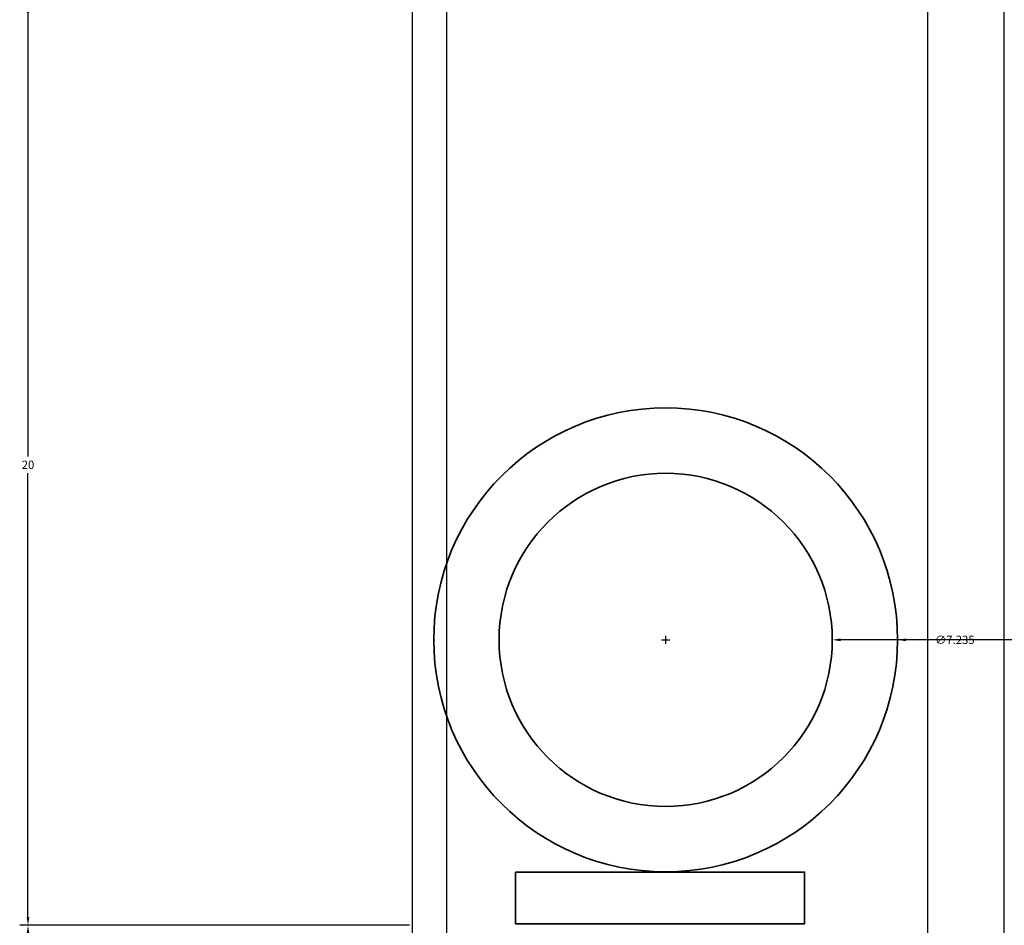
# Model space of a CAD drawing. Units: millimetres. Extents: x 446512 to 447461, y 70395 to 70610.
# Tile 13 of 39: x 446678.04 to 446699.43, y 70493.38 to 70513.05. Entities that reach past the tile are written whole.
import ezdxf

# ---------------------------------------------------------------- set-up
doc = ezdxf.new("R2010")
doc.units = ezdxf.units.MM
doc.layers.add('A-ANNO-DIMS', color=2, linetype='Continuous', lineweight=18)
doc.layers.add('A-FURN', color=7, linetype='Continuous', lineweight=35)
doc.styles.get("Standard").update_dxf_attribs({"font": 'arial.ttf'})
doc.dimstyles.get("Standard").update_dxf_attribs({"dimtxt": 0.18, "dimasz": 0.18, "dimexe": 0.18, "dimexo": 0.0625, "dimgap": 0.09, "dimtad": 0, "dimtih": 1, "dimtoh": 1, "dimdec": 4, "dimzin": 0, "dimdsep": 46, "dimtxsty": 'Standard', "dimcen": 0.09, "dimadec": 0, "dimazin": 0, "dimtfac": 1, "dimtdec": 4, "dimtofl": 0, "dimtmove": 0, "dimatfit": 3, "dimfxl": 1, "dimtolj": 1, "dimtzin": 0, "dimarcsym": 0})

# ---------------------------------------------------------------- blocks, each defined once
blk = doc.blocks.new('*D21')
at = {"layer": 'A-ANNO-DIMS', "color": 0, "lineweight": -2, "transparency": 16777216}
for p, q in [((446686.51, 70493.382), (446678.043, 70493.382)), ((446678.223, 70493.202), (446678.223, 70483.563)), ((446678.223, 70473.562), (446678.223, 70483.2)), ((446686.51, 70473.382), (446678.043, 70473.382))]:
    blk.add_line(p, q, dxfattribs=at)
at = {"layer": 'A-ANNO-DIMS', "color": 0, "transparency": 16777216}
for points in [[(446678.193, 70493.202), (446678.253, 70493.202), (446678.223, 70493.382)], [(446678.193, 70473.562), (446678.253, 70473.562), (446678.223, 70473.382)]]:
    blk.add_solid(points, dxfattribs=at)
at = {"layer": 'Defpoints', "color": 0, "transparency": 16777216}
for p in [(446678.223, 70493.382), (446686.573, 70493.382), (446686.573, 70473.382)]:
    blk.add_point(p, dxfattribs=at)
at = {"layer": 'A-ANNO-DIMS', "color": 0, "transparency": 16777216, "insert": (446678.223, 70483.382), "char_height": 0.18, "attachment_point": 5}
blk.add_mtext('\\A1;20', dxfattribs=at)
blk = doc.blocks.new('*D22')
at = {"layer": 'A-ANNO-DIMS', "color": 0, "lineweight": -2, "transparency": 16777216}
for p, q in [((446686.51, 70513.382), (446678.043, 70513.382)), ((446678.223, 70513.202), (446678.223, 70503.563)), ((446678.223, 70493.562), (446678.223, 70503.2)), ((446686.51, 70493.382), (446678.043, 70493.382))]:
    blk.add_line(p, q, dxfattribs=at)
at = {"layer": 'A-ANNO-DIMS', "color": 0, "transparency": 16777216}
for points in [[(446678.193, 70513.202), (446678.253, 70513.202), (446678.223, 70513.382)], [(446678.193, 70493.562), (446678.253, 70493.562), (446678.223, 70493.382)]]:
    blk.add_solid(points, dxfattribs=at)
at = {"layer": 'Defpoints', "color": 0, "transparency": 16777216}
for p in [(446678.223, 70513.382), (446686.573, 70513.382), (446686.573, 70493.382)]:
    blk.add_point(p, dxfattribs=at)
at = {"layer": 'A-ANNO-DIMS', "color": 0, "transparency": 16777216, "insert": (446678.223, 70503.382), "char_height": 0.18, "attachment_point": 5}
blk.add_mtext('\\A1;20', dxfattribs=at)
blk = doc.blocks.new('*D37')
at = {"layer": 'A-ANNO-DIMS', "color": 0, "lineweight": -2, "transparency": 16777216}
for p, q in [((446686.572846, 70433.44405), (446686.572846, 70578.17492)), ((446687.323552, 70428.838404), (446687.323552, 70578.17492)), ((446686.392846, 70577.99492), (446686.212846, 70577.99492)), ((446687.503552, 70577.99492), (446687.683552, 70577.99492))]:
    blk.add_line(p, q, dxfattribs=at)
at = {"layer": 'A-ANNO-DIMS', "color": 0, "transparency": 16777216}
for points in [[(446686.392846, 70578.02492), (446686.392846, 70577.96492), (446686.572846, 70577.99492)], [(446687.503552, 70578.02492), (446687.503552, 70577.96492), (446687.323552, 70577.99492)]]:
    blk.add_solid(points, dxfattribs=at)
at = {"layer": 'Defpoints', "color": 0, "transparency": 16777216}
for p in [(446687.323552, 70577.99492), (446686.572846, 70433.38155), (446687.323552, 70428.775904)]:
    blk.add_point(p, dxfattribs=at)
at = {"layer": 'A-ANNO-DIMS', "color": 0, "transparency": 16777216, "insert": (446686.948199, 70577.99492), "char_height": 0.18, "attachment_point": 5}
blk.add_mtext('\\A1;0.75', dxfattribs=at)
blk = doc.blocks.new('*D38')
at = {"layer": 'A-ANNO-DIMS', "color": 0, "lineweight": -2, "transparency": 16777216}
for p, q in [((446687.323552, 70428.838404), (446687.323552, 70578.17492)), ((446697.765686, 70428.838404), (446697.765686, 70578.17492)), ((446687.503552, 70577.99492), (446692.090383, 70577.99492)), ((446697.585686, 70577.99492), (446692.998855, 70577.99492))]:
    blk.add_line(p, q, dxfattribs=at)
at = {"layer": 'A-ANNO-DIMS', "color": 0, "transparency": 16777216}
for points in [[(446687.503552, 70578.02492), (446687.503552, 70577.96492), (446687.323552, 70577.99492)], [(446697.585686, 70578.02492), (446697.585686, 70577.96492), (446697.765686, 70577.99492)]]:
    blk.add_solid(points, dxfattribs=at)
at = {"layer": 'Defpoints', "color": 0, "transparency": 16777216}
for p in [(446697.765686, 70577.99492), (446687.323552, 70428.775904), (446697.765686, 70428.775904)]:
    blk.add_point(p, dxfattribs=at)
at = {"layer": 'A-ANNO-DIMS', "color": 0, "transparency": 16777216, "insert": (446692.544619, 70577.99492), "char_height": 0.18, "attachment_point": 5}
blk.add_mtext('\\A1;10.442', dxfattribs=at)
blk = doc.blocks.new('*D39')
at = {"layer": 'A-ANNO-DIMS', "color": 0, "lineweight": -2, "transparency": 16777216}
for p, q in [((446697.766, 70428.838), (446697.766, 70578.175)), ((446699.429, 70433.444), (446699.429, 70578.175)), ((446697.946, 70577.995), (446698.212, 70577.995)), ((446699.249, 70577.995), (446698.982, 70577.995))]:
    blk.add_line(p, q, dxfattribs=at)
at = {"layer": 'A-ANNO-DIMS', "color": 0, "transparency": 16777216}
for points in [[(446697.946, 70578.025), (446697.946, 70577.965), (446697.766, 70577.995)], [(446699.249, 70578.025), (446699.249, 70577.965), (446699.429, 70577.995)]]:
    blk.add_solid(points, dxfattribs=at)
at = {"layer": 'Defpoints', "color": 0, "transparency": 16777216}
for p in [(446699.429, 70577.995), (446699.429, 70433.382), (446697.766, 70428.776)]:
    blk.add_point(p, dxfattribs=at)
at = {"layer": 'A-ANNO-DIMS', "color": 0, "transparency": 16777216, "insert": (446698.597, 70577.995), "char_height": 0.18, "attachment_point": 5}
blk.add_mtext('\\A1;1.663', dxfattribs=at)
blk = doc.blocks.new('*D75')
at = {"layer": 'A-ANNO-DIMS', "color": 0, "lineweight": -2, "transparency": 16777216}
for p, q in [((446691.984, 70499.581), (446692.164, 70499.581)), ((446692.074, 70499.491), (446692.074, 70499.671)), ((446700.134, 70499.581), (446697.291, 70499.581))]:
    blk.add_line(p, q, dxfattribs=at)
at = {"layer": 'A-ANNO-DIMS', "color": 0, "transparency": 16777216}
blk.add_solid([(446697.291, 70499.611), (446697.291, 70499.551), (446697.111, 70499.581)], dxfattribs=at)
at = {"layer": 'Defpoints', "color": 0, "transparency": 16777216}
for p in [(446687.036, 70499.58), (446697.111, 70499.581)]:
    blk.add_point(p, dxfattribs=at)
at = {"layer": 'A-ANNO-DIMS', "color": 0, "transparency": 16777216, "insert": (446700.696, 70499.581), "char_height": 0.18, "attachment_point": 5}
blk.add_mtext('\\A1;∅10.075', dxfattribs=at)
blk = doc.blocks.new('*D76')
at = {"layer": 'A-ANNO-DIMS', "color": 0, "lineweight": -2, "transparency": 16777216}
for p, q in [((446691.984, 70499.581), (446692.164, 70499.581)), ((446692.074, 70499.491), (446692.074, 70499.671)), ((446697.862, 70499.581), (446695.871, 70499.581))]:
    blk.add_line(p, q, dxfattribs=at)
at = {"layer": 'A-ANNO-DIMS', "color": 0, "transparency": 16777216}
blk.add_solid([(446695.871, 70499.611), (446695.871, 70499.551), (446695.691, 70499.581)], dxfattribs=at)
at = {"layer": 'Defpoints', "color": 0, "transparency": 16777216}
for p in [(446688.456, 70499.58), (446695.691, 70499.581)]:
    blk.add_point(p, dxfattribs=at)
at = {"layer": 'A-ANNO-DIMS', "color": 0, "transparency": 16777216, "insert": (446698.354, 70499.581), "char_height": 0.18, "attachment_point": 5}
blk.add_mtext('\\A1;∅7.235', dxfattribs=at)

msp = doc.modelspace()

# ---------------------------------------------------------------- linework, layer by layer
at = {"layer": 'A-FURN'}
msp.add_lwpolyline([(446688.812, 70494.5368), (446695.0924, 70494.5368), (446695.0924, 70493.416), (446688.812, 70493.416)], close=True, dxfattribs=at)
for radius in [5.0377, 3.6176]:
    msp.add_circle((446692.0736, 70499.5807), radius, dxfattribs=at)

# ---------------------------------------------------------------- dimensions: what is measured, and where the dimension line sits
at = {"layer": 'A-ANNO-DIMS'}
for base, p1, p2, override, picture, middle in [((446687.3236, 70577.9949), (446686.5728, 70433.3816), (446687.3236, 70428.7759), {"dimdec": 2, "dimlfac": 1, "dimrnd": 0, "dimzin": 0, "dimdsep": 46, "dimlunit": 2}, '*D37', (446686.9482, 70577.9949)), ((446697.7657, 70577.9949), (446687.3236, 70428.7759), (446697.7657, 70428.7759), {"dimdec": 3, "dimlfac": 1, "dimrnd": 0, "dimzin": 0, "dimdsep": 46, "dimlunit": 2}, '*D38', (446692.5446, 70577.9949)), ((446699.4288, 70577.9949), (446697.7657, 70428.7759), (446699.4288, 70433.3816), {"dimdec": 3, "dimlfac": 1, "dimrnd": 0, "dimzin": 0, "dimdsep": 46, "dimlunit": 2}, '*D39', (446698.5973, 70577.9949))]:
    dim = msp.add_linear_dim(base=base, p1=p1, p2=p2, dimstyle='Standard', override=override, dxfattribs=at)
    dim.commit()
    dim.dimension.update_dxf_attribs({"geometry": picture, "text_midpoint": middle})
for base, p1, p2, picture, middle in [((446678.2228, 70513.3816), (446686.5728, 70493.3816), (446686.5728, 70513.3816), '*D22', (446678.2228, 70503.3815)), ((446678.2228, 70493.3816), (446686.5728, 70473.3816), (446686.5728, 70493.3816), '*D21', (446678.2228, 70483.3815))]:
    dim = msp.add_linear_dim(base=base, p1=p1, p2=p2, angle=90, dimstyle='Standard', override={"dimdec": 0, "dimlfac": 1, "dimrnd": 0, "dimzin": 0, "dimdsep": 46, "dimlunit": 2}, dxfattribs=at)
    dim.commit()
    dim.dimension.update_dxf_attribs({"geometry": picture, "text_midpoint": middle})
for p1, p2, picture, middle in [((446687.0359, 70499.5805), (446697.1113, 70499.581), '*D75', (446700.134, 70499.5812)), ((446688.456, 70499.5805), (446695.6912, 70499.581), '*D76', (446697.8617, 70499.5812))]:
    dim = msp.add_diameter_dim_2p(p1=p1, p2=p2, dimstyle='Standard', override={"dimdec": 3, "dimlfac": 1, "dimrnd": 0, "dimzin": 0, "dimdsep": 46, "dimlunit": 2}, dxfattribs=at)
    dim.commit()
    dim.dimension.update_dxf_attribs({"geometry": picture, "text_midpoint": middle, "dimtype": 163})

doc.saveas('drawing.dxf')
